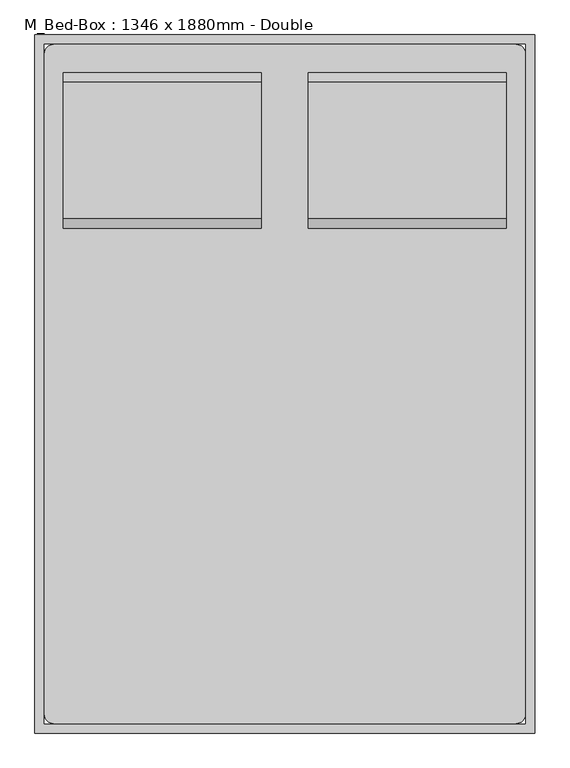
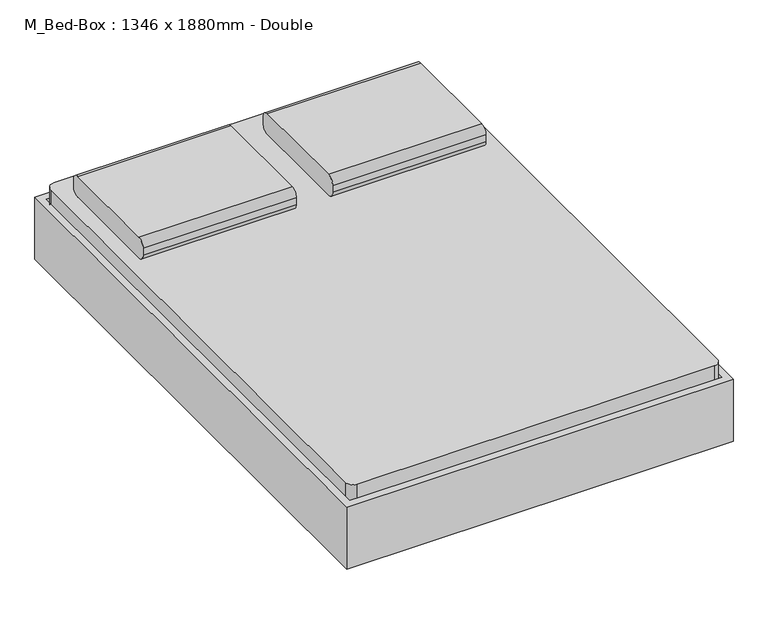
"""IFC4 building model written with IfcOpenShell, lengths in millimetres: furniture geometry, M_Bed-Box : 1346 x 1880mm - Double."""

from ifc_helpers import new_model, si_unit, point, frame, frame_2d, origin, place, context, project, spatial, polyline, circle_curve, trimmed, segment, composite_curve, outline, extrude, source, transform, mapped, element, save
from ifc_brep_helpers import plane_surface, cylinder_surface, revolved_surface, advanced_brep


def m_bed_box_1346_x_1880mm_double_b32eb57e(model_context):
    return source(origin(), model_context, "Body", "SolidModel", [
        extrude(outline(composite_curve([segment(polyline([(578.5704918, 406.4), (210.2704918, 406.4)]), True, "CONTINUOUS"), segment(trimmed(circle_curve(frame_2d((210.2704918, 431.8)), 25.4), [point((210.2704918, 406.4))], [point((184.8704918, 431.8))], False, "CARTESIAN"), True, "CONTINUOUS"), segment(polyline([(184.8704918, 431.8), (184.8704918, 457.2)]), True, "CONTINUOUS"), segment(trimmed(circle_curve(frame_2d((210.2704918, 457.2)), 25.4), [point((184.8704918, 457.2))], [point((210.2704918, 482.6))], False, "CARTESIAN"), True, "CONTINUOUS"), segment(polyline([(210.2704918, 482.6), (578.5704918, 482.6)]), True, "CONTINUOUS"), segment(trimmed(circle_curve(frame_2d((578.5704918, 457.2)), 25.4), [point((578.5704918, 482.6))], [point((603.9704918, 457.2))], False, "CARTESIAN"), True, "CONTINUOUS"), segment(polyline([(603.9704918, 457.2), (603.9704918, 431.8)]), True, "CONTINUOUS"), segment(trimmed(circle_curve(frame_2d((578.5704918, 431.8)), 25.4), [point((603.9704918, 431.8))], [point((578.5704918, 406.4))], False, "CARTESIAN"), True, "CONTINUOUS")], self_intersect=False)), frame((402.652459, 0.0, 0.0), z_axis=(1.0, 0.0, 0.0), x_axis=(0.0, 1.0, 0.0)), (0.0, 0.0, 1.0), 533.3),
        extrude(outline(composite_curve([segment(polyline([(578.5704918, 406.4), (210.2704918, 406.4)]), True, "CONTINUOUS"), segment(trimmed(circle_curve(frame_2d((210.2704918, 431.8)), 25.4), [point((210.2704918, 406.4))], [point((184.8704918, 431.8))], False, "CARTESIAN"), True, "CONTINUOUS"), segment(polyline([(184.8704918, 431.8), (184.8704918, 457.2)]), True, "CONTINUOUS"), segment(trimmed(circle_curve(frame_2d((210.2704918, 457.2)), 25.4), [point((184.8704918, 457.2))], [point((210.2704918, 482.6))], False, "CARTESIAN"), True, "CONTINUOUS"), segment(polyline([(210.2704918, 482.6), (578.5704918, 482.6)]), True, "CONTINUOUS"), segment(trimmed(circle_curve(frame_2d((578.5704918, 457.2)), 25.4), [point((578.5704918, 482.6))], [point((603.9704918, 457.2))], False, "CARTESIAN"), True, "CONTINUOUS"), segment(polyline([(603.9704918, 457.2), (603.9704918, 431.8)]), True, "CONTINUOUS"), segment(trimmed(circle_curve(frame_2d((578.5704918, 431.8)), 25.4), [point((603.9704918, 431.8))], [point((578.5704918, 406.4))], False, "CARTESIAN"), True, "CONTINUOUS")], self_intersect=False)), frame((-257.647541, 0.0, 0.0), z_axis=(1.0, 0.0, 0.0), x_axis=(0.0, 1.0, 0.0)), (0.0, 0.0, 1.0), 533.3),
        advanced_brep(
        [(-308.1231784, 451.5704918, 177.8), (-308.1231784, 375.3704918, 177.8), (-308.1231784, 375.3704918, 196.85), (-308.1231784, 451.5704918, 196.85), (-257.3231784, 451.5704918, 177.8), (-257.3231784, 375.3704918, 177.8), (-245.1869899, 375.3704918, 196.85), (-245.1869899, 451.5704918, 196.85), (-181.2523099, 451.5704918, 14.6654962), (-181.2523099, 375.3704918, 14.6654962), (-163.9871466, 375.3704918, 22.716374), (-163.9871466, 451.5704918, 22.716374), (-158.2320921, 375.3704918, 0.0), (-158.2320921, 451.5704918, 0.0), (-158.2320921, 375.3704918, 19.05), (-158.2320921, 451.5704918, 19.05), (-79.6195862, 451.5704918, 0.0), (-79.6195862, 375.3704918, 0.0), (-79.6195862, 375.3704918, 19.05), (-79.6195862, 451.5704918, 19.05), (-66.9195862, 375.3704918, 3.4029547), (-66.9195862, 451.5704918, 3.4029547), (-76.4445862, 375.3704918, 19.9007387), (-76.4445862, 451.5704918, 19.9007387), (-6.822541, 451.5704918, 38.1), (-6.822541, 375.3704918, 38.1), (-11.9269731, 375.3704918, 57.15), (-11.9269731, 451.5704918, 57.15), (685.4518216, 451.5704918, 38.1), (685.4518216, 375.3704918, 38.1), (690.5562537, 375.3704918, 57.15), (690.5562537, 451.5704918, 57.15), (745.5488669, 451.5704918, 3.4029547), (745.5488669, 375.3704918, 3.4029547), (755.0738669, 375.3704918, 19.9007387), (755.0738669, 451.5704918, 19.9007387), (758.2488669, 375.3704918, 0.0), (758.2488669, 451.5704918, 0.0), (758.2488669, 375.3704918, 19.05), (758.2488669, 451.5704918, 19.05), (836.8613728, 451.5704918, 0.0), (836.8613728, 375.3704918, 0.0), (836.8613728, 375.3704918, 19.05), (836.8613728, 451.5704918, 19.05), (859.8815906, 375.3704918, 14.6654962), (859.8815906, 451.5704918, 14.6654962), (842.6164272, 375.3704918, 22.716374), (842.6164272, 451.5704918, 22.716374), (935.952459, 451.5704918, 177.8), (935.952459, 375.3704918, 177.8), (923.8162705, 375.3704918, 196.85), (923.8162705, 451.5704918, 196.85), (986.752459, 451.5704918, 177.8), (986.752459, 451.5704918, 196.85), (986.752459, 375.3704918, 196.85), (986.752459, 375.3704918, 177.8)],
        [
            (0, 1),
            (1, 2),
            (2, 3),
            (3, 0),
            (0, 4),
            (4, 5),
            (5, 1),
            (5, 6),
            (6, 2),
            (6, 7),
            (7, 3),
            (7, 4),
            (4, 8),
            (8, 9),
            (9, 5),
            (9, 10),
            (10, 6),
            (10, 11),
            (11, 7),
            (11, 8),
            (12, 9, circle_curve(frame((-158.2320921, 375.3704918, 25.4), z_axis=(0.0, 1.0, 0.0), x_axis=(-0.906307787036649, 0.0, -0.4226182617407015)), 25.4)),
            (8, 13, circle_curve(frame((-158.2320921, 451.5704918, 25.4), z_axis=(0.0, -1.0, 0.0), x_axis=(-0.906307787036649, 0.0, -0.4226182617407015)), 25.4)),
            (13, 12),
            (14, 10, circle_curve(frame((-158.2320921, 375.3704918, 25.4), z_axis=(0.0, 1.0, 0.0), x_axis=(-0.906307787036649, 0.0, -0.4226182617407015)), 6.35)),
            (12, 14),
            (15, 11, circle_curve(frame((-158.2320921, 451.5704918, 25.4), z_axis=(0.0, 1.0, 0.0), x_axis=(-0.906307787036649, 0.0, -0.4226182617407015)), 6.35)),
            (14, 15),
            (15, 13),
            (13, 16),
            (16, 17),
            (17, 12),
            (17, 18),
            (18, 14),
            (18, 19),
            (19, 15),
            (19, 16),
            (20, 17, circle_curve(frame((-79.6195862, 375.3704918, 25.4), z_axis=(0.0, 1.0, 0.0), x_axis=(0.0, 0.0, -1.0)), 25.4)),
            (16, 21, circle_curve(frame((-79.6195862, 451.5704918, 25.4), z_axis=(0.0, -1.0, 0.0), x_axis=(0.0, 0.0, -1.0)), 25.4)),
            (21, 20),
            (22, 18, circle_curve(frame((-79.6195862, 375.3704918, 25.4), z_axis=(0.0, 1.0, 0.0), x_axis=(0.0, 0.0, -1.0)), 6.35)),
            (20, 22),
            (23, 19, circle_curve(frame((-79.6195862, 451.5704918, 25.4), z_axis=(0.0, 1.0, 0.0), x_axis=(0.0, 0.0, -1.0)), 6.35)),
            (22, 23),
            (23, 21),
            (21, 24),
            (24, 25),
            (25, 20),
            (25, 26),
            (26, 22),
            (26, 27),
            (27, 23),
            (27, 24),
            (24, 28),
            (28, 29),
            (29, 25),
            (29, 30),
            (30, 26),
            (30, 31),
            (31, 27),
            (31, 28),
            (28, 32),
            (32, 33),
            (33, 29),
            (33, 34),
            (34, 30),
            (34, 35),
            (35, 31),
            (35, 32),
            (36, 33, circle_curve(frame((758.2488669, 375.3704918, 25.4), z_axis=(0.0, 1.0, 0.0), x_axis=(-0.5000000000000463, 0.0, -0.8660254037844118)), 25.4)),
            (32, 37, circle_curve(frame((758.2488669, 451.5704918, 25.4), z_axis=(0.0, -1.0, 0.0), x_axis=(-0.5000000000000463, 0.0, -0.8660254037844118)), 25.4)),
            (37, 36),
            (38, 34, circle_curve(frame((758.2488669, 375.3704918, 25.4), z_axis=(0.0, 1.0, 0.0), x_axis=(-0.5000000000000463, 0.0, -0.8660254037844118)), 6.35)),
            (36, 38),
            (39, 35, circle_curve(frame((758.2488669, 451.5704918, 25.4), z_axis=(0.0, 1.0, 0.0), x_axis=(-0.5000000000000463, 0.0, -0.8660254037844118)), 6.35)),
            (38, 39),
            (39, 37),
            (37, 40),
            (40, 41),
            (41, 36),
            (41, 42),
            (42, 38),
            (42, 43),
            (43, 39),
            (43, 40),
            (44, 41, circle_curve(frame((836.8613728, 375.3704918, 25.4), z_axis=(0.0, 1.0, 0.0), x_axis=(0.0, 0.0, -1.0)), 25.4)),
            (40, 45, circle_curve(frame((836.8613728, 451.5704918, 25.4), z_axis=(0.0, -1.0, 0.0), x_axis=(0.0, 0.0, -1.0)), 25.4)),
            (45, 44),
            (46, 42, circle_curve(frame((836.8613728, 375.3704918, 25.4), z_axis=(0.0, 1.0, 0.0), x_axis=(0.0, 0.0, -1.0)), 6.35)),
            (44, 46),
            (47, 43, circle_curve(frame((836.8613728, 451.5704918, 25.4), z_axis=(0.0, 1.0, 0.0), x_axis=(0.0, 0.0, -1.0)), 6.35)),
            (46, 47),
            (47, 45),
            (45, 48),
            (48, 49),
            (49, 44),
            (49, 50),
            (50, 46),
            (50, 51),
            (51, 47),
            (51, 48),
            (52, 53),
            (53, 54),
            (54, 55),
            (55, 52),
            (48, 52),
            (55, 49),
            (54, 50),
            (53, 51),
        ],
        [
            plane_surface(frame((-308.1231784, 705.5704918, -152.9490627), z_axis=(-1.0, 0.0, 0.0), x_axis=(0.0, 1.0, 0.0))),
            plane_surface(frame((-308.1231784, 451.5704918, 177.8), z_axis=(0.0, 0.0, -1.0), x_axis=(1.0, 0.0, 0.0))),
            plane_surface(frame((-308.1231784, 375.3704918, 177.8), z_axis=(0.0, -1.0, 0.0), x_axis=(1.0, 0.0, 0.0))),
            plane_surface(frame((-308.1231784, 375.3704918, 196.85), z_axis=(0.0, 0.0, 1.0), x_axis=(1.0, 0.0, 0.0))),
            plane_surface(frame((-308.1231784, 451.5704918, 196.85), z_axis=(0.0, 1.0, 0.0), x_axis=(1.0, 0.0, 0.0))),
            plane_surface(frame((-257.3231784, 451.5704918, 177.8), z_axis=(-0.9063077870366486, 0.0, -0.4226182617407026), x_axis=(0.4226182617407026, 0.0, -0.9063077870366486))),
            plane_surface(frame((-257.3231784, 375.3704918, 177.8), z_axis=(0.0, -1.0000000000000002, 0.0), x_axis=(0.4226182617407026, 0.0, -0.9063077870366486))),
            plane_surface(frame((-245.1869899, 375.3704918, 196.85), z_axis=(0.9063077870366487, 0.0, 0.4226182617407023), x_axis=(0.4226182617407023, 0.0, -0.9063077870366487))),
            plane_surface(frame((-245.1869899, 451.5704918, 196.85), z_axis=(0.0, 1.0, 0.0), x_axis=(0.4226182617407027, 0.0, -0.9063077870366485))),
            cylinder_surface(frame((-158.2320921, 705.5704918, 25.4), z_axis=(0.0, -1.0, 0.0), x_axis=(-0.906307787036649, 0.0, -0.4226182617407015)), 25.4),
            plane_surface(frame((-158.2320921, 375.3704918, 25.4), z_axis=(0.0, -1.0, 0.0), x_axis=(-0.906307787036649, 0.0, -0.4226182617407015))),
            revolved_surface(polyline([(-163.9871465476827, 375.3704918, 22.716374037946544), (-163.9871465476827, 451.5704918, 22.716374037946544)]), (-158.2320921, 705.5704918, 25.4), (0.0, -1.0, 0.0)),
            plane_surface(frame((-158.2320921, 451.5704918, 25.4), z_axis=(0.0, 1.0, 0.0), x_axis=(-0.906307787036649, 0.0, -0.4226182617407015))),
            plane_surface(frame((-158.2320921, 451.5704918, 0.0), z_axis=(0.0, 0.0, -1.0), x_axis=(1.0, 0.0, 0.0))),
            plane_surface(frame((-158.2320921, 375.3704918, 0.0), z_axis=(0.0, -1.0, 0.0), x_axis=(1.0, 0.0, 0.0))),
            plane_surface(frame((-158.2320921, 375.3704918, 19.05), z_axis=(0.0, 0.0, 1.0), x_axis=(1.0, 0.0, 0.0))),
            plane_surface(frame((-158.2320921, 451.5704918, 19.05), z_axis=(0.0, 1.0, 0.0), x_axis=(1.0, 0.0, 0.0))),
            cylinder_surface(frame((-79.6195862, 705.5704918, 25.4), z_axis=(0.0, -1.0, 0.0), x_axis=(0.0, 0.0, -1.0)), 25.4),
            plane_surface(frame((-79.6195862, 375.3704918, 25.4), z_axis=(0.0, -1.0, 0.0), x_axis=(0.0, 0.0, -1.0))),
            revolved_surface(polyline([(-79.6195862, 375.3704918, 19.049999999999997), (-79.6195862, 451.5704918, 19.049999999999997)]), (-79.6195862, 705.5704918, 25.4), (0.0, -1.0, 0.0)),
            plane_surface(frame((-79.6195862, 451.5704918, 25.4), z_axis=(0.0, 1.0, 0.0), x_axis=(0.0, 0.0, -1.0))),
            plane_surface(frame((-66.9195862, 451.5704918, 3.4029547), z_axis=(0.4999999999998744, 0.0, -0.8660254037845112), x_axis=(0.8660254037845112, 0.0, 0.4999999999998744))),
            plane_surface(frame((-66.9195862, 375.3704918, 3.4029547), z_axis=(0.0, -1.0000000000000002, 0.0), x_axis=(0.8660254037845112, 0.0, 0.4999999999998745))),
            plane_surface(frame((-76.4445862, 375.3704918, 19.9007387), z_axis=(-0.4999999999998741, 0.0, 0.8660254037845113), x_axis=(0.8660254037845113, 0.0, 0.4999999999998741))),
            plane_surface(frame((-76.4445862, 451.5704918, 19.9007387), z_axis=(0.0, 1.0, 0.0), x_axis=(0.866025403784511, 0.0, 0.49999999999987477))),
            plane_surface(frame((-6.822541, 451.5704918, 38.1), z_axis=(0.0, 0.0, -1.0), x_axis=(1.0, 0.0, 0.0))),
            plane_surface(frame((-6.822541, 375.3704918, 38.1), z_axis=(0.0, -1.0, 0.0), x_axis=(1.0, 0.0, 0.0))),
            plane_surface(frame((-11.9269731, 375.3704918, 57.15), z_axis=(0.0, 0.0, 1.0), x_axis=(1.0, 0.0, 0.0))),
            plane_surface(frame((-11.9269731, 451.5704918, 57.15), z_axis=(0.0, 1.0, 0.0), x_axis=(1.0, 0.0, 0.0))),
            plane_surface(frame((685.4518216, 451.5704918, 38.1), z_axis=(-0.5000000000000494, 0.0, -0.8660254037844102), x_axis=(0.8660254037844102, 0.0, -0.5000000000000494))),
            plane_surface(frame((685.4518216, 375.3704918, 38.1), z_axis=(0.0, -1.0, 0.0), x_axis=(0.8660254037844112, 0.0, -0.5000000000000476))),
            plane_surface(frame((690.5562537, 375.3704918, 57.15), z_axis=(0.5000000000000488, 0.0, 0.8660254037844105), x_axis=(0.8660254037844105, 0.0, -0.5000000000000488))),
            plane_surface(frame((690.5562537, 451.5704918, 57.15), z_axis=(0.0, 1.0, 0.0), x_axis=(0.8660254037844106, 0.0, -0.5000000000000485))),
            cylinder_surface(frame((758.2488669, 705.5704918, 25.4), z_axis=(0.0, -1.0, 0.0), x_axis=(-0.5000000000000463, 0.0, -0.8660254037844118)), 25.4),
            plane_surface(frame((758.2488669, 375.3704918, 25.4), z_axis=(0.0, -1.0000000000000002, 0.0), x_axis=(-0.5000000000000464, 0.0, -0.866025403784412))),
            revolved_surface(polyline([(755.0738668999998, 375.3704918, 19.90073868596898), (755.0738668999998, 451.5704918, 19.90073868596898)]), (758.2488669, 705.5704918, 25.4), (0.0, -1.0, 0.0)),
            plane_surface(frame((758.2488669, 451.5704918, 25.4), z_axis=(0.0, 1.0000000000000002, 0.0), x_axis=(-0.5000000000000464, 0.0, -0.866025403784412))),
            plane_surface(frame((758.2488669, 451.5704918, 0.0), z_axis=(0.0, 0.0, -1.0), x_axis=(1.0, 0.0, 0.0))),
            plane_surface(frame((758.2488669, 375.3704918, 0.0), z_axis=(0.0, -1.0, 0.0), x_axis=(1.0, 0.0, 0.0))),
            plane_surface(frame((758.2488669, 375.3704918, 19.05), z_axis=(0.0, 0.0, 1.0), x_axis=(1.0, 0.0, 0.0))),
            plane_surface(frame((758.2488669, 451.5704918, 19.05), z_axis=(0.0, 1.0, 0.0), x_axis=(1.0, 0.0, 0.0))),
            cylinder_surface(frame((836.8613728, 705.5704918, 25.4), z_axis=(0.0, -1.0, 0.0), x_axis=(0.0, 0.0, -1.0)), 25.4),
            plane_surface(frame((836.8613728, 375.3704918, 25.4), z_axis=(0.0, -1.0, 0.0), x_axis=(0.0, 0.0, -1.0))),
            revolved_surface(polyline([(836.8613728, 375.3704918, 19.049999999999997), (836.8613728, 451.5704918, 19.049999999999997)]), (836.8613728, 705.5704918, 25.4), (0.0, -1.0, 0.0)),
            plane_surface(frame((836.8613728, 451.5704918, 25.4), z_axis=(0.0, 1.0, 0.0), x_axis=(0.0, 0.0, -1.0))),
            plane_surface(frame((859.8815906, 451.5704918, 14.6654962), z_axis=(0.90630778703668, 0.0, -0.422618261740635), x_axis=(0.422618261740635, 0.0, 0.90630778703668))),
            plane_surface(frame((859.8815906, 375.3704918, 14.6654962), z_axis=(0.0, -1.0000000000000002, 0.0), x_axis=(0.4226182617406349, 0.0, 0.9063077870366801))),
            plane_surface(frame((842.6164272, 375.3704918, 22.716374), z_axis=(-0.9063077870366805, 0.0, 0.4226182617406341), x_axis=(0.4226182617406341, 0.0, 0.9063077870366805))),
            plane_surface(frame((842.6164272, 451.5704918, 22.716374), z_axis=(0.0, 1.0, 0.0), x_axis=(0.42261826174063455, 0.0, 0.9063077870366802))),
            plane_surface(frame((986.752459, 705.5704918, -152.9490627), z_axis=(1.0, 0.0, 0.0), x_axis=(0.0, 1.0, 0.0))),
            plane_surface(frame((935.952459, 451.5704918, 177.8), z_axis=(0.0, 0.0, -1.0), x_axis=(1.0, 0.0, 0.0))),
            plane_surface(frame((935.952459, 375.3704918, 177.8), z_axis=(0.0, -1.0, 0.0), x_axis=(1.0, 0.0, 0.0))),
            plane_surface(frame((923.8162705, 375.3704918, 196.85), z_axis=(0.0, 0.0, 1.0), x_axis=(1.0, 0.0, 0.0))),
            plane_surface(frame((923.8162705, 451.5704918, 196.85), z_axis=(0.0, 1.0, 0.0), x_axis=(1.0, 0.0, 0.0))),
        ],
        [
            (0, [[1, 2, 3, 4]]),
            (1, [[-1, 5, 6, 7]]),
            (2, [[-2, -7, 8, 9]]),
            (3, [[-3, -9, 10, 11]]),
            (4, [[-4, -11, 12, -5]]),
            (5, [[-6, 13, 14, 15]]),
            (6, [[-8, -15, 16, 17]]),
            (7, [[-10, -17, 18, 19]]),
            (8, [[-12, -19, 20, -13]]),
            (9, [[21, -14, 22, 23]]),
            (10, [[24, -16, -21, 25]]),
            (11, [[26, -18, -24, 27]]),
            (12, [[-22, -20, -26, 28]]),
            (13, [[-23, 29, 30, 31]]),
            (14, [[-25, -31, 32, 33]]),
            (15, [[-27, -33, 34, 35]]),
            (16, [[-28, -35, 36, -29]]),
            (17, [[37, -30, 38, 39]]),
            (18, [[40, -32, -37, 41]]),
            (19, [[42, -34, -40, 43]]),
            (20, [[-38, -36, -42, 44]]),
            (21, [[-39, 45, 46, 47]]),
            (22, [[-41, -47, 48, 49]]),
            (23, [[-43, -49, 50, 51]]),
            (24, [[-44, -51, 52, -45]]),
            (25, [[-46, 53, 54, 55]]),
            (26, [[-48, -55, 56, 57]]),
            (27, [[-50, -57, 58, 59]]),
            (28, [[-52, -59, 60, -53]]),
            (29, [[-54, 61, 62, 63]]),
            (30, [[-56, -63, 64, 65]]),
            (31, [[-58, -65, 66, 67]]),
            (32, [[-60, -67, 68, -61]]),
            (33, [[69, -62, 70, 71]]),
            (34, [[72, -64, -69, 73]]),
            (35, [[74, -66, -72, 75]]),
            (36, [[-70, -68, -74, 76]]),
            (37, [[-71, 77, 78, 79]]),
            (38, [[-73, -79, 80, 81]]),
            (39, [[-75, -81, 82, 83]]),
            (40, [[-76, -83, 84, -77]]),
            (41, [[85, -78, 86, 87]]),
            (42, [[88, -80, -85, 89]]),
            (43, [[90, -82, -88, 91]]),
            (44, [[-86, -84, -90, 92]]),
            (45, [[-87, 93, 94, 95]]),
            (46, [[-89, -95, 96, 97]]),
            (47, [[-91, -97, 98, 99]]),
            (48, [[-92, -99, 100, -93]]),
            (49, [[101, 102, 103, 104]]),
            (50, [[-94, 105, -104, 106]]),
            (51, [[-96, -106, -103, 107]]),
            (52, [[-98, -107, -102, 108]]),
            (53, [[-100, -108, -101, -105]]),
        ],
    ),
        extrude(outline(composite_curve([segment(polyline([(-283.047541, 680.1704918), (961.352459, 680.1704918)]), True, "CONTINUOUS"), segment(trimmed(circle_curve(frame_2d((961.352459, 654.7704918)), 25.4), [point((961.352459, 680.1704918))], [point((986.752459, 654.7704918))], False, "CARTESIAN"), True, "CONTINUOUS"), segment(polyline([(986.752459, 654.7704918), (986.752459, -1123.6295082)]), True, "CONTINUOUS"), segment(trimmed(circle_curve(frame_2d((961.352459, -1123.6295082)), 25.4), [point((986.752459, -1123.6295082))], [point((961.352459, -1149.0295082))], False, "CARTESIAN"), True, "CONTINUOUS"), segment(polyline([(961.352459, -1149.0295082), (-283.047541, -1149.0295082)]), True, "CONTINUOUS"), segment(trimmed(circle_curve(frame_2d((-283.047541, -1123.6295082)), 25.4), [point((-283.047541, -1149.0295082))], [point((-308.447541, -1123.6295082))], False, "CARTESIAN"), True, "CONTINUOUS"), segment(polyline([(-308.447541, -1123.6295082), (-308.447541, 654.7704918)]), True, "CONTINUOUS"), segment(trimmed(circle_curve(frame_2d((-283.047541, 654.7704918)), 25.4), [point((-308.447541, 654.7704918))], [point((-283.047541, 680.1704918))], False, "CARTESIAN"), True, "CONTINUOUS")], self_intersect=False)), frame((0.0, 0.0, 203.2), z_axis=(0.0, 0.0, 1.0), x_axis=(1.0, 0.0, 0.0)), (0.0, 0.0, 1.0), 203.2),
        advanced_brep(
        [(-308.447541, -869.6295082, 196.85), (-308.447541, -869.6295082, 177.8), (-308.447541, -945.8295082, 177.8), (-308.447541, -945.8295082, 196.85), (-245.5113525, -869.6295082, 196.85), (-257.647541, -869.6295082, 177.8), (-257.647541, -945.8295082, 177.8), (-245.5113525, -945.8295082, 196.85), (-164.3115092, -869.6295082, 22.716374), (-181.5766725, -869.6295082, 14.6654962), (-181.5766725, -945.8295082, 14.6654962), (-164.3115092, -945.8295082, 22.716374), (-158.5564547, -869.6295082, 0.0), (-158.5564547, -869.6295082, 19.05), (-158.5564547, -945.8295082, 0.0), (-158.5564547, -945.8295082, 19.05), (-79.9439489, -869.6295082, 19.05), (-79.9439489, -869.6295082, 0.0), (-79.9439489, -945.8295082, 0.0), (-79.9439489, -945.8295082, 19.05), (-67.2439489, -869.6295082, 3.4029547), (-76.7689489, -869.6295082, 19.9007387), (-67.2439489, -945.8295082, 3.4029547), (-76.7689489, -945.8295082, 19.9007387), (-12.2513357, -869.6295082, 57.15), (-7.1469036, -869.6295082, 38.1), (-7.1469036, -945.8295082, 38.1), (-12.2513357, -945.8295082, 57.15), (690.5562537, -869.6295082, 57.15), (685.4518216, -869.6295082, 38.1), (685.4518216, -945.8295082, 38.1), (690.5562537, -945.8295082, 57.15), (755.0738669, -869.6295082, 19.9007387), (745.5488669, -869.6295082, 3.4029547), (745.5488669, -945.8295082, 3.4029547), (755.0738669, -945.8295082, 19.9007387), (758.2488669, -869.6295082, 0.0), (758.2488669, -869.6295082, 19.05), (758.2488669, -945.8295082, 0.0), (758.2488669, -945.8295082, 19.05), (836.8613728, -869.6295082, 19.05), (836.8613728, -869.6295082, 0.0), (836.8613728, -945.8295082, 0.0), (836.8613728, -945.8295082, 19.05), (859.8815906, -869.6295082, 14.6654962), (842.6164272, -869.6295082, 22.716374), (859.8815906, -945.8295082, 14.6654962), (842.6164272, -945.8295082, 22.716374), (923.8162705, -869.6295082, 196.85), (935.952459, -869.6295082, 177.8), (935.952459, -945.8295082, 177.8), (923.8162705, -945.8295082, 196.85), (986.752459, -869.6295082, 196.85), (986.752459, -945.8295082, 196.85), (986.752459, -945.8295082, 177.8), (986.752459, -869.6295082, 177.8)],
        [
            (0, 1),
            (1, 2),
            (2, 3),
            (3, 0),
            (0, 4),
            (4, 5),
            (5, 1),
            (5, 6),
            (6, 2),
            (6, 7),
            (7, 3),
            (7, 4),
            (4, 8),
            (8, 9),
            (9, 5),
            (9, 10),
            (10, 6),
            (10, 11),
            (11, 7),
            (11, 8),
            (12, 9, circle_curve(frame((-158.5564547, -869.6295082, 25.4), z_axis=(0.0, 1.0, 0.0), x_axis=(-0.9063077870366625, 0.0, -0.4226182617406725)), 25.4)),
            (8, 13, circle_curve(frame((-158.5564547, -869.6295082, 25.4), z_axis=(0.0, -1.0, 0.0), x_axis=(-0.9063077870366625, 0.0, -0.4226182617406725)), 6.35)),
            (13, 12),
            (14, 10, circle_curve(frame((-158.5564547, -945.8295082, 25.4), z_axis=(0.0, 1.0, 0.0), x_axis=(-0.9063077870366625, 0.0, -0.4226182617406725)), 25.4)),
            (12, 14),
            (15, 11, circle_curve(frame((-158.5564547, -945.8295082, 25.4), z_axis=(0.0, 1.0, 0.0), x_axis=(-0.9063077870366625, 0.0, -0.4226182617406725)), 6.35)),
            (14, 15),
            (15, 13),
            (13, 16),
            (16, 17),
            (17, 12),
            (17, 18),
            (18, 14),
            (18, 19),
            (19, 15),
            (19, 16),
            (20, 17, circle_curve(frame((-79.9439489, -869.6295082, 25.4), z_axis=(0.0, 1.0, 0.0), x_axis=(0.0, 0.0, -1.0)), 25.4)),
            (16, 21, circle_curve(frame((-79.9439489, -869.6295082, 25.4), z_axis=(0.0, -1.0, 0.0), x_axis=(0.0, 0.0, -1.0)), 6.35)),
            (21, 20),
            (22, 18, circle_curve(frame((-79.9439489, -945.8295082, 25.4), z_axis=(0.0, 1.0, 0.0), x_axis=(0.0, 0.0, -1.0)), 25.4)),
            (20, 22),
            (23, 19, circle_curve(frame((-79.9439489, -945.8295082, 25.4), z_axis=(0.0, 1.0, 0.0), x_axis=(0.0, 0.0, -1.0)), 6.35)),
            (22, 23),
            (23, 21),
            (21, 24),
            (24, 25),
            (25, 20),
            (25, 26),
            (26, 22),
            (26, 27),
            (27, 23),
            (27, 24),
            (24, 28),
            (28, 29),
            (29, 25),
            (29, 30),
            (30, 26),
            (30, 31),
            (31, 27),
            (31, 28),
            (28, 32),
            (32, 33),
            (33, 29),
            (33, 34),
            (34, 30),
            (34, 35),
            (35, 31),
            (35, 32),
            (36, 33, circle_curve(frame((758.2488669, -869.6295082, 25.4), z_axis=(0.0, 1.0, 0.0), x_axis=(-0.5000000000000528, 0.0, -0.8660254037844081)), 25.4)),
            (32, 37, circle_curve(frame((758.2488669, -869.6295082, 25.4), z_axis=(0.0, -1.0, 0.0), x_axis=(-0.5000000000000528, 0.0, -0.8660254037844081)), 6.35)),
            (37, 36),
            (38, 34, circle_curve(frame((758.2488669, -945.8295082, 25.4), z_axis=(0.0, 1.0, 0.0), x_axis=(-0.5000000000000528, 0.0, -0.8660254037844081)), 25.4)),
            (36, 38),
            (39, 35, circle_curve(frame((758.2488669, -945.8295082, 25.4), z_axis=(0.0, 1.0, 0.0), x_axis=(-0.5000000000000528, 0.0, -0.8660254037844081)), 6.35)),
            (38, 39),
            (39, 37),
            (37, 40),
            (40, 41),
            (41, 36),
            (41, 42),
            (42, 38),
            (42, 43),
            (43, 39),
            (43, 40),
            (44, 41, circle_curve(frame((836.8613728, -869.6295082, 25.4), z_axis=(0.0, 1.0, 0.0), x_axis=(0.0, 0.0, -1.0)), 25.4)),
            (40, 45, circle_curve(frame((836.8613728, -869.6295082, 25.4), z_axis=(0.0, -1.0, 0.0), x_axis=(0.0, 0.0, -1.0)), 6.35)),
            (45, 44),
            (46, 42, circle_curve(frame((836.8613728, -945.8295082, 25.4), z_axis=(0.0, 1.0, 0.0), x_axis=(0.0, 0.0, -1.0)), 25.4)),
            (44, 46),
            (47, 43, circle_curve(frame((836.8613728, -945.8295082, 25.4), z_axis=(0.0, 1.0, 0.0), x_axis=(0.0, 0.0, -1.0)), 6.35)),
            (46, 47),
            (47, 45),
            (45, 48),
            (48, 49),
            (49, 44),
            (49, 50),
            (50, 46),
            (50, 51),
            (51, 47),
            (51, 48),
            (52, 53),
            (53, 54),
            (54, 55),
            (55, 52),
            (48, 52),
            (55, 49),
            (54, 50),
            (53, 51),
        ],
        [
            plane_surface(frame((-308.447541, -1174.4295082, -127.5947323), z_axis=(-1.0, 0.0, 0.0), x_axis=(0.0, 1.0, 0.0))),
            plane_surface(frame((-308.447541, -869.6295082, 196.85), z_axis=(0.0, 1.0, 0.0), x_axis=(1.0, 0.0, 0.0))),
            plane_surface(frame((-308.447541, -869.6295082, 177.8), z_axis=(0.0, 0.0, -1.0), x_axis=(1.0, 0.0, 0.0))),
            plane_surface(frame((-308.447541, -945.8295082, 177.8), z_axis=(0.0, -1.0, 0.0), x_axis=(1.0, 0.0, 0.0))),
            plane_surface(frame((-308.447541, -945.8295082, 196.85), z_axis=(0.0, 0.0, 1.0), x_axis=(1.0, 0.0, 0.0))),
            plane_surface(frame((-245.5113525, -869.6295082, 196.85), z_axis=(0.0, 1.0, 0.0), x_axis=(0.4226182617406714, 0.0, -0.906307787036663))),
            plane_surface(frame((-257.647541, -869.6295082, 177.8), z_axis=(-0.9063077870366631, 0.0, -0.42261826174067146), x_axis=(0.42261826174067146, 0.0, -0.9063077870366631))),
            plane_surface(frame((-257.647541, -945.8295082, 177.8), z_axis=(0.0, -1.0000000000000002, 0.0), x_axis=(0.4226182617406716, 0.0, -0.906307787036663))),
            plane_surface(frame((-245.5113525, -945.8295082, 196.85), z_axis=(0.906307787036663, 0.0, 0.4226182617406716), x_axis=(0.4226182617406716, 0.0, -0.906307787036663))),
            plane_surface(frame((-158.5564547, -869.6295082, 25.4), z_axis=(0.0, 1.0, 0.0), x_axis=(-0.9063077870366625, 0.0, -0.4226182617406725))),
            cylinder_surface(frame((-158.5564547, -1174.4295082, 25.4), z_axis=(0.0, -1.0, 0.0), x_axis=(-0.9063077870366625, 0.0, -0.4226182617406725)), 25.4),
            plane_surface(frame((-158.5564547, -945.8295082, 25.4), z_axis=(0.0, -1.0, 0.0), x_axis=(-0.9063077870366625, 0.0, -0.4226182617406725))),
            revolved_surface(polyline([(-164.31150914768278, -945.8295082, 22.71637403794673), (-164.31150914768278, -869.6295082, 22.71637403794673)]), (-158.5564547, -1174.4295082, 25.4), (0.0, -1.0, 0.0)),
            plane_surface(frame((-158.5564547, -869.6295082, 19.05), z_axis=(0.0, 1.0, 0.0), x_axis=(1.0, 0.0, 0.0))),
            plane_surface(frame((-158.5564547, -869.6295082, 0.0), z_axis=(0.0, 0.0, -1.0), x_axis=(1.0, 0.0, 0.0))),
            plane_surface(frame((-158.5564547, -945.8295082, 0.0), z_axis=(0.0, -1.0, 0.0), x_axis=(1.0, 0.0, 0.0))),
            plane_surface(frame((-158.5564547, -945.8295082, 19.05), z_axis=(0.0, 0.0, 1.0), x_axis=(1.0, 0.0, 0.0))),
            plane_surface(frame((-79.9439489, -869.6295082, 25.4), z_axis=(0.0, 1.0, 0.0), x_axis=(0.0, 0.0, -1.0))),
            cylinder_surface(frame((-79.9439489, -1174.4295082, 25.4), z_axis=(0.0, -1.0, 0.0), x_axis=(0.0, 0.0, -1.0)), 25.4),
            plane_surface(frame((-79.9439489, -945.8295082, 25.4), z_axis=(0.0, -1.0, 0.0), x_axis=(0.0, 0.0, -1.0))),
            revolved_surface(polyline([(-79.9439489, -945.8295082, 19.049999999999997), (-79.9439489, -869.6295082, 19.049999999999997)]), (-79.9439489, -1174.4295082, 25.4), (0.0, -1.0, 0.0)),
            plane_surface(frame((-76.7689489, -869.6295082, 19.9007387), z_axis=(0.0, 1.0000000000000002, 0.0), x_axis=(0.8660254037844788, 0.0, 0.49999999999993067))),
            plane_surface(frame((-67.2439489, -869.6295082, 3.4029547), z_axis=(0.49999999999993067, 0.0, -0.8660254037844787), x_axis=(0.8660254037844787, 0.0, 0.49999999999993067))),
            plane_surface(frame((-67.2439489, -945.8295082, 3.4029547), z_axis=(0.0, -1.0, 0.0), x_axis=(0.8660254037844782, 0.0, 0.4999999999999315))),
            plane_surface(frame((-76.7689489, -945.8295082, 19.9007387), z_axis=(-0.49999999999993044, 0.0, 0.8660254037844789), x_axis=(0.8660254037844789, 0.0, 0.49999999999993044))),
            plane_surface(frame((-12.2513357, -869.6295082, 57.15), z_axis=(0.0, 1.0, 0.0), x_axis=(1.0, 0.0, 0.0))),
            plane_surface(frame((-7.1469036, -869.6295082, 38.1), z_axis=(0.0, 0.0, -1.0), x_axis=(1.0, 0.0, 0.0))),
            plane_surface(frame((-7.1469036, -945.8295082, 38.1), z_axis=(0.0, -1.0, 0.0), x_axis=(1.0, 0.0, 0.0))),
            plane_surface(frame((-12.2513357, -945.8295082, 57.15), z_axis=(0.0, 0.0, 1.0), x_axis=(1.0, 0.0, 0.0))),
            plane_surface(frame((690.5562537, -869.6295082, 57.15), z_axis=(0.0, 1.0, 0.0), x_axis=(0.8660254037844087, 0.0, -0.5000000000000518))),
            plane_surface(frame((685.4518216, -869.6295082, 38.1), z_axis=(-0.5000000000000513, 0.0, -0.8660254037844092), x_axis=(0.8660254037844092, 0.0, -0.5000000000000513))),
            plane_surface(frame((685.4518216, -945.8295082, 38.1), z_axis=(0.0, -1.0, 0.0), x_axis=(0.8660254037844081, 0.0, -0.5000000000000531))),
            plane_surface(frame((690.5562537, -945.8295082, 57.15), z_axis=(0.5000000000000521, 0.0, 0.8660254037844086), x_axis=(0.8660254037844086, 0.0, -0.5000000000000521))),
            plane_surface(frame((758.2488669, -869.6295082, 25.4), z_axis=(0.0, 1.0000000000000002, 0.0), x_axis=(-0.500000000000053, 0.0, -0.8660254037844082))),
            cylinder_surface(frame((758.2488669, -1174.4295082, 25.4), z_axis=(0.0, -1.0, 0.0), x_axis=(-0.5000000000000528, 0.0, -0.8660254037844081)), 25.4),
            plane_surface(frame((758.2488669, -945.8295082, 25.4), z_axis=(0.0, -1.0000000000000002, 0.0), x_axis=(-0.500000000000053, 0.0, -0.8660254037844082))),
            revolved_surface(polyline([(755.0738668999998, -945.8295082, 19.900738685969007), (755.0738668999998, -869.6295082, 19.900738685969007)]), (758.2488669, -1174.4295082, 25.4), (0.0, -1.0, 0.0)),
            plane_surface(frame((758.2488669, -869.6295082, 19.05), z_axis=(0.0, 1.0, 0.0), x_axis=(1.0, 0.0, 0.0))),
            plane_surface(frame((758.2488669, -869.6295082, 0.0), z_axis=(0.0, 0.0, -1.0), x_axis=(1.0, 0.0, 0.0))),
            plane_surface(frame((758.2488669, -945.8295082, 0.0), z_axis=(0.0, -1.0, 0.0), x_axis=(1.0, 0.0, 0.0))),
            plane_surface(frame((758.2488669, -945.8295082, 19.05), z_axis=(0.0, 0.0, 1.0), x_axis=(1.0, 0.0, 0.0))),
            plane_surface(frame((836.8613728, -869.6295082, 25.4), z_axis=(0.0, 1.0, 0.0), x_axis=(0.0, 0.0, -1.0))),
            cylinder_surface(frame((836.8613728, -1174.4295082, 25.4), z_axis=(0.0, -1.0, 0.0), x_axis=(0.0, 0.0, -1.0)), 25.4),
            plane_surface(frame((836.8613728, -945.8295082, 25.4), z_axis=(0.0, -1.0, 0.0), x_axis=(0.0, 0.0, -1.0))),
            revolved_surface(polyline([(836.8613728, -945.8295082, 19.049999999999997), (836.8613728, -869.6295082, 19.049999999999997)]), (836.8613728, -1174.4295082, 25.4), (0.0, -1.0, 0.0)),
            plane_surface(frame((842.6164272, -869.6295082, 22.716374), z_axis=(0.0, 1.0, 0.0), x_axis=(0.4226182617405387, 0.0, 0.906307787036725))),
            plane_surface(frame((859.8815906, -869.6295082, 14.6654962), z_axis=(0.906307787036725, 0.0, -0.4226182617405386), x_axis=(0.4226182617405386, 0.0, 0.906307787036725))),
            plane_surface(frame((859.8815906, -945.8295082, 14.6654962), z_axis=(0.0, -1.0, 0.0), x_axis=(0.4226182617405387, 0.0, 0.906307787036725))),
            plane_surface(frame((842.6164272, -945.8295082, 22.716374), z_axis=(-0.9063077870367251, 0.0, 0.4226182617405384), x_axis=(0.4226182617405384, 0.0, 0.9063077870367251))),
            plane_surface(frame((986.752459, -1174.4295082, -127.5947323), z_axis=(1.0, 0.0, 0.0), x_axis=(0.0, 1.0, 0.0))),
            plane_surface(frame((923.8162705, -869.6295082, 196.85), z_axis=(0.0, 1.0, 0.0), x_axis=(1.0, 0.0, 0.0))),
            plane_surface(frame((935.952459, -869.6295082, 177.8), z_axis=(0.0, 0.0, -1.0), x_axis=(1.0, 0.0, 0.0))),
            plane_surface(frame((935.952459, -945.8295082, 177.8), z_axis=(0.0, -1.0, 0.0), x_axis=(1.0, 0.0, 0.0))),
            plane_surface(frame((923.8162705, -945.8295082, 196.85), z_axis=(0.0, 0.0, 1.0), x_axis=(1.0, 0.0, 0.0))),
        ],
        [
            (0, [[1, 2, 3, 4]]),
            (1, [[-1, 5, 6, 7]]),
            (2, [[-2, -7, 8, 9]]),
            (3, [[-3, -9, 10, 11]]),
            (4, [[-4, -11, 12, -5]]),
            (5, [[-6, 13, 14, 15]]),
            (6, [[-8, -15, 16, 17]]),
            (7, [[-10, -17, 18, 19]]),
            (8, [[-12, -19, 20, -13]]),
            (9, [[21, -14, 22, 23]]),
            (10, [[24, -16, -21, 25]]),
            (11, [[26, -18, -24, 27]]),
            (12, [[-22, -20, -26, 28]]),
            (13, [[-23, 29, 30, 31]]),
            (14, [[-25, -31, 32, 33]]),
            (15, [[-27, -33, 34, 35]]),
            (16, [[-28, -35, 36, -29]]),
            (17, [[37, -30, 38, 39]]),
            (18, [[40, -32, -37, 41]]),
            (19, [[42, -34, -40, 43]]),
            (20, [[-38, -36, -42, 44]]),
            (21, [[-39, 45, 46, 47]]),
            (22, [[-41, -47, 48, 49]]),
            (23, [[-43, -49, 50, 51]]),
            (24, [[-44, -51, 52, -45]]),
            (25, [[-46, 53, 54, 55]]),
            (26, [[-48, -55, 56, 57]]),
            (27, [[-50, -57, 58, 59]]),
            (28, [[-52, -59, 60, -53]]),
            (29, [[-54, 61, 62, 63]]),
            (30, [[-56, -63, 64, 65]]),
            (31, [[-58, -65, 66, 67]]),
            (32, [[-60, -67, 68, -61]]),
            (33, [[69, -62, 70, 71]]),
            (34, [[72, -64, -69, 73]]),
            (35, [[74, -66, -72, 75]]),
            (36, [[-70, -68, -74, 76]]),
            (37, [[-71, 77, 78, 79]]),
            (38, [[-73, -79, 80, 81]]),
            (39, [[-75, -81, 82, 83]]),
            (40, [[-76, -83, 84, -77]]),
            (41, [[85, -78, 86, 87]]),
            (42, [[88, -80, -85, 89]]),
            (43, [[90, -82, -88, 91]]),
            (44, [[-86, -84, -90, 92]]),
            (45, [[-87, 93, 94, 95]]),
            (46, [[-89, -95, 96, 97]]),
            (47, [[-91, -97, 98, 99]]),
            (48, [[-92, -99, 100, -93]]),
            (49, [[101, 102, 103, 104]]),
            (50, [[-94, 105, -104, 106]]),
            (51, [[-96, -106, -103, 107]]),
            (52, [[-98, -107, -102, 108]]),
            (53, [[-100, -108, -101, -105]]),
        ],
    ),
        extrude(outline(polyline([(1012.152459, 705.5704918), (1012.152459, -1174.4295082), (-333.847541, -1174.4295082), (-333.847541, 705.5704918), (1012.152459, 705.5704918)]), holes=[polyline([(986.752459, 680.1704918), (-308.447541, 680.1704918), (-308.447541, -1149.0295082), (986.752459, -1149.0295082), (986.752459, 680.1704918)])]), frame((0.0, 0.0, 127.0), z_axis=(0.0, 0.0, 1.0), x_axis=(1.0, 0.0, 0.0)), (0.0, 0.0, 1.0), 228.6),
    ])


if __name__ == "__main__":
    model = new_model("IFC4")
    model_context = context("Model", 3, world=origin())
    ifc_project = project(units=[si_unit("LENGTHUNIT", "METRE", prefix="MILLI")], contexts=[model_context])
    site = spatial("IfcSite", under=ifc_project)
    building = spatial("IfcBuilding", under=site)
    placement = place(None, origin())
    m_bed_box_1346_x_1880mm_double_shape = m_bed_box_1346_x_1880mm_double_b32eb57e(model_context)
    element("IfcFurniture", 1, ObjectType="M_Bed-Box : 1346 x 1880mm - Double", at=placement, inside=building, context=model_context, shape_type="MappedRepresentation", body=[
        mapped(m_bed_box_1346_x_1880mm_double_shape, transform((0.0, 0.0, 0.0), x_axis=(1.0, 0.0, 0.0), y_axis=(0.0, 1.0, 0.0), z_axis=(0.0, 0.0, 1.0))),
    ])
    save(model, "model.ifc")

# Revit data of these elements
# Type "M_Bed-Box : 1346 x 1880mm - Double"
#   Length = 1880 mm
#   Width = 1346 mm
#   Frame Material = Birch
#   Mattress Material = Linen, White
#   Default Elevation = 0
# Element 1 (IfcFurniture, "M_Bed-Box : 1346 x 1880mm - Double")
#   Materials on its faces: "Birch", "Linen, White"
# Materials
#   "Birch": class "Wood", colour RGB 224 178 126, transparency 0, Description = "Betula Alleghaniensis", Cost = 0
#   "Linen, White": class "Textile", colour RGB 247 247 239, transparency 0, Description = "Linen, white", Cost = 0
